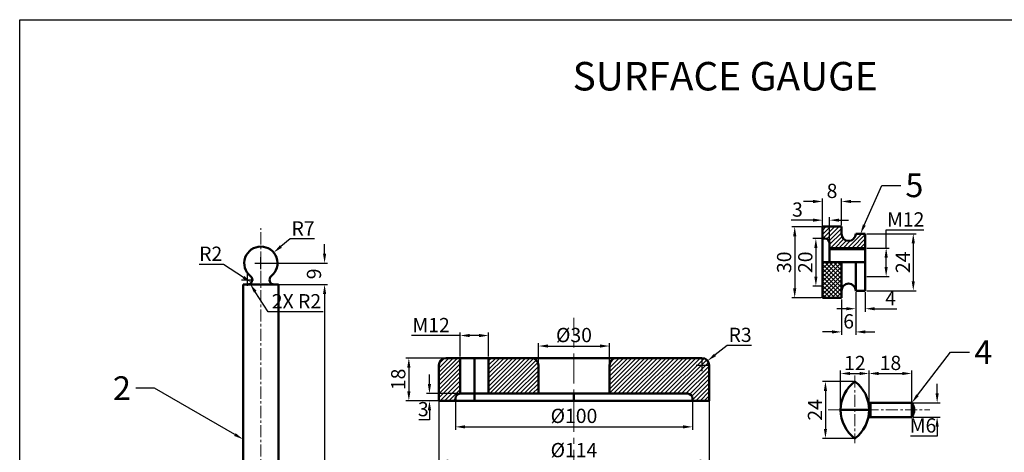
# Model space of a CAD drawing. Units: millimetres. Extents: x -65 to 576, y -103 to 374.
# Tile 3 of 4: x -65 to 351, y 192 to 374. Entities that reach past the tile are written whole.
import ezdxf
from ezdxf import colors
from ezdxf.entities.mleader import LeaderData, LeaderLine
from ezdxf.math import Vec2, Vec3

# ---------------------------------------------------------------- set-up
doc = ezdxf.new("R2010")
doc.units = ezdxf.units.MM
doc.header["$LTSCALE"] = 0.4
doc.linetypes.add('CENTER', pattern=[50.8, 31.75, -6.35, 6.35, -6.35])
for name, color, linetype, lineweight in [('M-CNTR', 4, 'CENTER', 18), ('M-DIMS', 2, 'Continuous', 25), ('M-HATC', 8, 'Continuous', 18), ('M-OUTL', 7, 'Continuous', 50), ('M-TEXT', 3, 'Continuous', 25), ('M-TTLB', 7, 'Continuous', 25)]:
    doc.layers.add(name, color=color, linetype=linetype, lineweight=lineweight)
doc.styles.get("Standard").update_dxf_attribs({"font": 'arial.ttf'})
doc.dimstyles.new('ISO-25', dxfattribs={"dimtxt": 6, "dimasz": 4, "dimexe": 1.25, "dimexo": 0.625, "dimtad": 1, "dimtoh": 1, "dimtxsty": 'Standard', "dimcen": 2.5, "dimadec": 0, "dimazin": 0, "dimtfac": 1, "dimtofl": 0, "dimtmove": 0, "dimatfit": 3, "dimfxl": 1, "dimarcsym": 0})

# ---------------------------------------------------------------- blocks, each defined once
blk = doc.blocks.new('*D1')
at = {"layer": 'Defpoints', "color": 0, "ltscale": 0.4, "transparency": 16777216}
for p in [(112.15, 220.83), (226.15, 220.83), (226.15, 187.9)]:
    blk.add_point(p, dxfattribs=at)
at = {"layer": 'M-DIMS', "color": 0, "lineweight": -2, "ltscale": 0.4, "transparency": 16777216}
for p, q in [((112.15, 220.2), (112.15, 186.65)), ((226.15, 220.2), (226.15, 186.65)), ((116.15, 187.9), (222.15, 187.9))]:
    blk.add_line(p, q, dxfattribs=at)
at = {"layer": 'M-DIMS', "color": 0, "ltscale": 0.4, "transparency": 16777216}
for points in [[(116.15, 188.57), (116.15, 187.24), (112.15, 187.9)], [(222.15, 188.57), (222.15, 187.24), (226.15, 187.9)]]:
    blk.add_solid(points, dxfattribs=at)
at = {"layer": 'M-DIMS', "color": 0, "ltscale": 0.4, "transparency": 16777216, "insert": (169.15, 191.76), "char_height": 6, "attachment_point": 5}
blk.add_mtext('%%C114', dxfattribs=at)
blk = doc.blocks.new('*D2')
at = {"layer": 'Defpoints', "color": 0, "ltscale": 0.4, "transparency": 16777216}
for p in [(119.15, 213.33), (219.15, 213.33), (219.15, 202.34)]:
    blk.add_point(p, dxfattribs=at)
at = {"layer": 'M-DIMS', "color": 0, "lineweight": -2, "ltscale": 0.4, "transparency": 16777216}
for p, q in [((119.15, 212.7), (119.15, 201.09)), ((219.15, 212.7), (219.15, 201.09)), ((123.15, 202.34), (215.15, 202.34))]:
    blk.add_line(p, q, dxfattribs=at)
at = {"layer": 'M-DIMS', "color": 0, "ltscale": 0.4, "transparency": 16777216}
for points in [[(123.15, 203), (123.15, 201.67), (119.15, 202.34)], [(215.15, 203), (215.15, 201.67), (219.15, 202.34)]]:
    blk.add_solid(points, dxfattribs=at)
at = {"layer": 'M-DIMS', "color": 0, "ltscale": 0.4, "transparency": 16777216, "insert": (169.15, 206.19), "char_height": 6, "attachment_point": 5}
blk.add_mtext('%%C100', dxfattribs=at)
blk = doc.blocks.new('*D3')
at = {"layer": 'Defpoints', "color": 0, "ltscale": 0.4, "transparency": 16777216}
for p in [(184.15, 236.39), (154.15, 222.33), (184.15, 222.33)]:
    blk.add_point(p, dxfattribs=at)
at = {"layer": 'M-DIMS', "color": 0, "lineweight": -2, "ltscale": 0.4, "transparency": 16777216}
for p, q in [((154.15, 222.95), (154.15, 237.64)), ((184.15, 222.95), (184.15, 237.64)), ((158.15, 236.39), (180.15, 236.39))]:
    blk.add_line(p, q, dxfattribs=at)
at = {"layer": 'M-DIMS', "color": 0, "ltscale": 0.4, "transparency": 16777216}
for points in [[(158.15, 237.05), (158.15, 235.72), (154.15, 236.39)], [(180.15, 237.05), (180.15, 235.72), (184.15, 236.39)]]:
    blk.add_solid(points, dxfattribs=at)
at = {"layer": 'M-DIMS', "color": 0, "ltscale": 0.4, "transparency": 16777216, "insert": (169.15, 240.24), "char_height": 6, "attachment_point": 5}
blk.add_mtext('%%C30', dxfattribs=at)
blk = doc.blocks.new('*D4')
at = {"layer": 'Defpoints', "color": 0, "ltscale": 0.4, "transparency": 16777216}
for p in [(133.15, 240.8), (121.15, 231.33), (133.15, 231.33)]:
    blk.add_point(p, dxfattribs=at)
at = {"layer": 'M-DIMS', "color": 0, "lineweight": -2, "ltscale": 0.4, "transparency": 16777216}
for p, q in [((121.15, 231.95), (121.15, 242.05)), ((133.15, 231.95), (133.15, 242.05)), ((121.15, 240.8), (100.65, 240.8)), ((129.15, 240.8), (125.15, 240.8))]:
    blk.add_line(p, q, dxfattribs=at)
at = {"layer": 'M-DIMS', "color": 0, "ltscale": 0.4, "transparency": 16777216}
for points in [[(125.15, 241.47), (125.15, 240.14), (121.15, 240.8)], [(129.15, 241.47), (129.15, 240.14), (133.15, 240.8)]]:
    blk.add_solid(points, dxfattribs=at)
at = {"layer": 'M-DIMS', "color": 0, "ltscale": 0.4, "transparency": 16777216, "insert": (108.9, 244.44), "char_height": 6, "attachment_point": 5}
blk.add_mtext('M12', dxfattribs=at)
blk = doc.blocks.new('*D5')
at = {"layer": 'Defpoints', "color": 0, "ltscale": 0.4, "transparency": 16777216}
for p in [(115.15, 231.33), (99.51, 213.33), (115.15, 213.33)]:
    blk.add_point(p, dxfattribs=at)
at = {"layer": 'M-DIMS', "color": 0, "lineweight": -2, "ltscale": 0.4, "transparency": 16777216}
for p, q in [((114.52, 231.33), (98.26, 231.33)), ((99.51, 227.33), (99.51, 217.33)), ((114.52, 213.33), (98.26, 213.33))]:
    blk.add_line(p, q, dxfattribs=at)
at = {"layer": 'M-DIMS', "color": 0, "ltscale": 0.4, "transparency": 16777216}
for points in [[(98.84, 227.33), (100.18, 227.33), (99.51, 231.33)], [(98.84, 217.33), (100.18, 217.33), (99.51, 213.33)]]:
    blk.add_solid(points, dxfattribs=at)
at = {"layer": 'M-DIMS', "color": 0, "ltscale": 0.4, "transparency": 16777216, "insert": (95.82, 222.33), "char_height": 6, "attachment_point": 5, "rotation": 90}
blk.add_mtext('18', dxfattribs=at)
blk = doc.blocks.new('*D6')
at = {"layer": 'Defpoints', "color": 0, "ltscale": 0.4, "transparency": 16777216}
for p in [(125.51, 216.33), (108.2, 213.33), (125.51, 213.33)]:
    blk.add_point(p, dxfattribs=at)
at = {"layer": 'M-DIMS', "color": 0, "lineweight": -2, "ltscale": 0.4, "transparency": 16777216}
for p, q in [((108.2, 220.33), (108.2, 224.33)), ((124.88, 216.33), (106.95, 216.33)), ((124.88, 213.33), (106.95, 213.33)), ((108.2, 209.33), (108.2, 205.33)), ((108.2, 205.33), (103.65, 205.33))]:
    blk.add_line(p, q, dxfattribs=at)
at = {"layer": 'M-DIMS', "color": 0, "ltscale": 0.4, "transparency": 16777216}
for points in [[(107.53, 220.33), (108.87, 220.33), (108.2, 216.33)], [(107.53, 209.33), (108.87, 209.33), (108.2, 213.33)]]:
    blk.add_solid(points, dxfattribs=at)
at = {"layer": 'M-DIMS', "color": 0, "ltscale": 0.4, "transparency": 16777216, "insert": (105.61, 209.02), "char_height": 6, "attachment_point": 5}
blk.add_mtext('3', dxfattribs=at)
blk = doc.blocks.new('*D7')
at = {"layer": 'Defpoints', "color": 0, "ltscale": 0.4, "transparency": 16777216}
for p in [(225.51, 230.18), (223.15, 228.33)]:
    blk.add_point(p, dxfattribs=at)
at = {"layer": 'M-DIMS', "color": 0, "lineweight": -2, "ltscale": 0.4, "transparency": 16777216}
for p, q in [((233.76, 236.63), (228.66, 232.64)), ((244.06, 236.63), (233.76, 236.63)), ((223.15, 225.83), (223.15, 230.83)), ((220.65, 228.33), (225.65, 228.33))]:
    blk.add_line(p, q, dxfattribs=at)
at = {"layer": 'M-DIMS', "color": 0, "ltscale": 0.4, "transparency": 16777216}
blk.add_solid([(228.25, 233.16), (229.07, 232.11), (225.51, 230.18)], dxfattribs=at)
at = {"layer": 'M-DIMS', "color": 0, "ltscale": 0.4, "transparency": 16777216, "insert": (239.22, 240.32), "char_height": 6, "attachment_point": 5}
blk.add_mtext('R3', dxfattribs=at)
blk = doc.blocks.new('*D12')
at = {"layer": 'Defpoints', "color": 0, "ltscale": 0.4, "transparency": 16777216}
for p in [(44.59, 262.28), (46.09, -30.72), (63.96, -30.72)]:
    blk.add_point(p, dxfattribs=at)
at = {"layer": 'M-DIMS', "color": 0, "lineweight": -2, "ltscale": 0.4, "transparency": 16777216}
for p, q in [((45.22, 262.28), (65.21, 262.28)), ((63.96, 258.28), (63.96, -26.72)), ((46.72, -30.72), (65.21, -30.72))]:
    blk.add_line(p, q, dxfattribs=at)
at = {"layer": 'M-DIMS', "color": 0, "ltscale": 0.4, "transparency": 16777216}
for points in [[(63.29, 258.28), (64.63, 258.28), (63.96, 262.28)], [(63.29, -26.72), (64.63, -26.72), (63.96, -30.72)]]:
    blk.add_solid(points, dxfattribs=at)
at = {"layer": 'M-DIMS', "color": 0, "ltscale": 0.4, "transparency": 16777216, "insert": (60.27, 115.78), "char_height": 6, "attachment_point": 5, "rotation": 90}
blk.add_mtext('293', dxfattribs=at)
blk = doc.blocks.new('*D17')
at = {"layer": 'Defpoints', "color": 0, "ltscale": 0.4, "transparency": 16777216}
for p in [(37.09, 271.28), (37.09, 262.28), (63.96, 262.28)]:
    blk.add_point(p, dxfattribs=at)
at = {"layer": 'M-DIMS', "color": 0, "lineweight": -2, "ltscale": 0.4, "transparency": 16777216}
for p, q in [((63.96, 275.28), (63.96, 279.28)), ((37.72, 271.28), (65.21, 271.28)), ((37.72, 262.28), (65.21, 262.28)), ((63.96, 258.28), (63.96, 254.28))]:
    blk.add_line(p, q, dxfattribs=at)
at = {"layer": 'M-DIMS', "color": 0, "ltscale": 0.4, "transparency": 16777216}
for points in [[(63.29, 275.28), (64.63, 275.28), (63.96, 271.28)], [(63.29, 258.28), (64.63, 258.28), (63.96, 262.28)]]:
    blk.add_solid(points, dxfattribs=at)
at = {"layer": 'M-DIMS', "color": 0, "ltscale": 0.4, "transparency": 16777216, "insert": (60.27, 266.78), "char_height": 6, "attachment_point": 5, "rotation": 90}
blk.add_mtext('9', dxfattribs=at)
blk = doc.blocks.new('*D18')
at = {"layer": 'Defpoints', "color": 0, "ltscale": 0.4, "transparency": 16777216}
for p in [(31.44, 264.28), (33.11, 263.19)]:
    blk.add_point(p, dxfattribs=at)
at = {"layer": 'M-DIMS', "color": 0, "lineweight": -2, "ltscale": 0.4, "transparency": 16777216}
for p, q in [((11.13, 270.85), (21.37, 270.85)), ((21.37, 270.85), (29.76, 265.37))]:
    blk.add_line(p, q, dxfattribs=at)
at = {"layer": 'M-DIMS', "color": 0, "ltscale": 0.4, "transparency": 16777216}
blk.add_solid([(30.13, 265.93), (29.4, 264.82), (33.11, 263.19)], dxfattribs=at)
at = {"layer": 'M-DIMS', "color": 0, "ltscale": 0.4, "transparency": 16777216, "insert": (15.94, 274.49), "char_height": 6, "attachment_point": 5}
blk.add_mtext('R2', dxfattribs=at)
blk = doc.blocks.new('*D19')
at = {"layer": 'Defpoints', "color": 0, "ltscale": 0.4, "transparency": 16777216}
for p in [(42.48, 275.75), (37.09, 271.28)]:
    blk.add_point(p, dxfattribs=at)
at = {"layer": 'M-DIMS', "color": 0, "lineweight": -2, "ltscale": 0.4, "transparency": 16777216}
for p, q in [((49.42, 281.51), (45.56, 278.3)), ((59.72, 281.51), (49.42, 281.51)), ((34.59, 271.28), (39.59, 271.28)), ((37.09, 268.78), (37.09, 273.78))]:
    blk.add_line(p, q, dxfattribs=at)
at = {"layer": 'M-DIMS', "color": 0, "ltscale": 0.4, "transparency": 16777216}
blk.add_solid([(45.13, 278.82), (45.98, 277.79), (42.48, 275.75)], dxfattribs=at)
at = {"layer": 'M-DIMS', "color": 0, "ltscale": 0.4, "transparency": 16777216, "insert": (54.89, 285.14), "char_height": 6, "attachment_point": 5}
blk.add_mtext('R7', dxfattribs=at)
blk = doc.blocks.new('*D20')
at = {"layer": 'Defpoints', "color": 0, "ltscale": 0.4, "transparency": 16777216}
for p in [(293.63, 224.81), (281.63, 209.48), (293.63, 209.48)]:
    blk.add_point(p, dxfattribs=at)
at = {"layer": 'M-DIMS', "color": 0, "lineweight": -2, "ltscale": 0.4, "transparency": 16777216}
for p, q in [((281.63, 210.1), (281.63, 226.06)), ((285.63, 224.81), (289.63, 224.81)), ((293.63, 210.1), (293.63, 226.06))]:
    blk.add_line(p, q, dxfattribs=at)
at = {"layer": 'M-DIMS', "color": 0, "ltscale": 0.4, "transparency": 16777216}
for points in [[(285.63, 225.48), (285.63, 224.15), (281.63, 224.81)], [(289.63, 225.48), (289.63, 224.15), (293.63, 224.81)]]:
    blk.add_solid(points, dxfattribs=at)
at = {"layer": 'M-DIMS', "color": 0, "ltscale": 0.4, "transparency": 16777216, "insert": (287.63, 228.45), "char_height": 6, "attachment_point": 5}
blk.add_mtext('12', dxfattribs=at)
blk = doc.blocks.new('*D21')
at = {"layer": 'Defpoints', "color": 0, "ltscale": 0.4, "transparency": 16777216}
for p in [(287.63, 221.48), (275.22, 197.48), (287.63, 197.48)]:
    blk.add_point(p, dxfattribs=at)
at = {"layer": 'M-DIMS', "color": 0, "lineweight": -2, "ltscale": 0.4, "transparency": 16777216}
for p, q in [((287, 221.48), (273.97, 221.48)), ((275.22, 217.48), (275.22, 201.48)), ((287, 197.48), (273.97, 197.48))]:
    blk.add_line(p, q, dxfattribs=at)
at = {"layer": 'M-DIMS', "color": 0, "ltscale": 0.4, "transparency": 16777216}
for points in [[(274.55, 217.48), (275.88, 217.48), (275.22, 221.48)], [(274.55, 201.48), (275.88, 201.48), (275.22, 197.48)]]:
    blk.add_solid(points, dxfattribs=at)
at = {"layer": 'M-DIMS', "color": 0, "ltscale": 0.4, "transparency": 16777216, "insert": (271.58, 209.48), "char_height": 6, "attachment_point": 5, "rotation": 90}
blk.add_mtext('24', dxfattribs=at)
blk = doc.blocks.new('*D22')
at = {"layer": 'Defpoints', "color": 0, "ltscale": 0.4, "transparency": 16777216}
for p in [(311.63, 212.48), (311.63, 206.48), (322.32, 206.48)]:
    blk.add_point(p, dxfattribs=at)
at = {"layer": 'M-DIMS', "color": 0, "lineweight": -2, "ltscale": 0.4, "transparency": 16777216}
for p, q in [((322.32, 216.48), (322.32, 220.48)), ((312.25, 212.48), (323.57, 212.48)), ((312.25, 206.48), (323.57, 206.48)), ((322.32, 202.48), (322.32, 198.48)), ((322.32, 198.48), (311.06, 198.48))]:
    blk.add_line(p, q, dxfattribs=at)
at = {"layer": 'M-DIMS', "color": 0, "ltscale": 0.4, "transparency": 16777216}
for points in [[(321.65, 216.48), (322.99, 216.48), (322.32, 212.48)], [(321.65, 202.48), (322.99, 202.48), (322.32, 206.48)]]:
    blk.add_solid(points, dxfattribs=at)
at = {"layer": 'M-DIMS', "color": 0, "ltscale": 0.4, "transparency": 16777216, "insert": (316.38, 202.16), "char_height": 6, "attachment_point": 5}
blk.add_mtext('M6', dxfattribs=at)
blk = doc.blocks.new('*D23')
at = {"layer": 'Defpoints', "color": 0, "ltscale": 0.4, "transparency": 16777216}
for p in [(311.63, 224.81), (293.63, 209.83), (311.63, 209.48)]:
    blk.add_point(p, dxfattribs=at)
at = {"layer": 'M-DIMS', "color": 0, "lineweight": -2, "ltscale": 0.4, "transparency": 16777216}
for p, q in [((293.63, 210.45), (293.63, 226.06)), ((297.63, 224.81), (307.63, 224.81)), ((311.63, 210.1), (311.63, 226.06))]:
    blk.add_line(p, q, dxfattribs=at)
at = {"layer": 'M-DIMS', "color": 0, "ltscale": 0.4, "transparency": 16777216}
for points in [[(297.63, 225.48), (297.63, 224.15), (293.63, 224.81)], [(307.63, 225.48), (307.63, 224.15), (311.63, 224.81)]]:
    blk.add_solid(points, dxfattribs=at)
at = {"layer": 'M-DIMS', "color": 0, "ltscale": 0.4, "transparency": 16777216, "insert": (302.63, 228.5), "char_height": 6, "attachment_point": 5}
blk.add_mtext('18', dxfattribs=at)
blk = doc.blocks.new('*D46')
at = {"layer": 'Defpoints', "color": 0, "ltscale": 0.4, "transparency": 16777216}
for p in [(273.99, 286.66), (262.25, 256.66), (273.99, 256.66)]:
    blk.add_point(p, dxfattribs=at)
at = {"layer": 'M-DIMS', "color": 0, "lineweight": -2, "ltscale": 0.4, "transparency": 16777216}
for p, q in [((273.36, 286.66), (261, 286.66)), ((262.25, 282.66), (262.25, 260.66)), ((273.36, 256.66), (261, 256.66))]:
    blk.add_line(p, q, dxfattribs=at)
at = {"layer": 'M-DIMS', "color": 0, "ltscale": 0.4, "transparency": 16777216}
for points in [[(261.59, 282.66), (262.92, 282.66), (262.25, 286.66)], [(261.59, 260.66), (262.92, 260.66), (262.25, 256.66)]]:
    blk.add_solid(points, dxfattribs=at)
at = {"layer": 'M-DIMS', "color": 0, "ltscale": 0.4, "transparency": 16777216, "insert": (258.56, 271.66), "char_height": 6, "attachment_point": 5, "rotation": 90}
blk.add_mtext('30', dxfattribs=at)
blk = doc.blocks.new('*D47')
at = {"layer": 'Defpoints', "color": 0, "ltscale": 0.4, "transparency": 16777216}
for p in [(273.99, 281.66), (271.18, 261.66), (274.49, 261.66)]:
    blk.add_point(p, dxfattribs=at)
at = {"layer": 'M-DIMS', "color": 0, "lineweight": -2, "ltscale": 0.4, "transparency": 16777216}
for p, q in [((273.36, 281.66), (269.93, 281.66)), ((271.18, 277.66), (271.18, 265.66)), ((273.86, 261.66), (269.93, 261.66))]:
    blk.add_line(p, q, dxfattribs=at)
at = {"layer": 'M-DIMS', "color": 0, "ltscale": 0.4, "transparency": 16777216}
for points in [[(270.51, 277.66), (271.85, 277.66), (271.18, 281.66)], [(270.51, 265.66), (271.85, 265.66), (271.18, 261.66)]]:
    blk.add_solid(points, dxfattribs=at)
at = {"layer": 'M-DIMS', "color": 0, "ltscale": 0.4, "transparency": 16777216, "insert": (267.49, 271.66), "char_height": 6, "attachment_point": 5, "rotation": 90}
blk.add_mtext('20', dxfattribs=at)
blk = doc.blocks.new('*D48')
at = {"layer": 'Defpoints', "color": 0, "ltscale": 0.4, "transparency": 16777216}
for p in [(281.99, 297.27), (273.99, 286.66), (281.99, 286.66)]:
    blk.add_point(p, dxfattribs=at)
at = {"layer": 'M-DIMS', "color": 0, "lineweight": -2, "ltscale": 0.4, "transparency": 16777216}
for p, q in [((269.99, 297.27), (265.99, 297.27)), ((273.99, 287.29), (273.99, 298.52)), ((281.99, 287.29), (281.99, 298.52)), ((285.99, 297.27), (289.99, 297.27))]:
    blk.add_line(p, q, dxfattribs=at)
at = {"layer": 'M-DIMS', "color": 0, "ltscale": 0.4, "transparency": 16777216}
for points in [[(269.99, 297.93), (269.99, 296.6), (273.99, 297.27)], [(285.99, 297.93), (285.99, 296.6), (281.99, 297.27)]]:
    blk.add_solid(points, dxfattribs=at)
at = {"layer": 'M-DIMS', "color": 0, "ltscale": 0.4, "transparency": 16777216, "insert": (277.99, 300.95), "char_height": 6, "attachment_point": 5}
blk.add_mtext('8', dxfattribs=at)
blk = doc.blocks.new('*D49')
at = {"layer": 'Defpoints', "color": 0, "ltscale": 0.4, "transparency": 16777216}
for p in [(276.99, 289.4), (273.99, 277.61), (276.99, 277.61)]:
    blk.add_point(p, dxfattribs=at)
at = {"layer": 'M-DIMS', "color": 0, "lineweight": -2, "ltscale": 0.4, "transparency": 16777216}
for p, q in [((269.99, 289.4), (260.81, 289.4)), ((273.99, 278.24), (273.99, 290.65)), ((276.99, 278.24), (276.99, 290.65)), ((280.99, 289.4), (284.99, 289.4))]:
    blk.add_line(p, q, dxfattribs=at)
at = {"layer": 'M-DIMS', "color": 0, "ltscale": 0.4, "transparency": 16777216}
for points in [[(269.99, 290.07), (269.99, 288.74), (273.99, 289.4)], [(280.99, 290.07), (280.99, 288.74), (276.99, 289.4)]]:
    blk.add_solid(points, dxfattribs=at)
at = {"layer": 'M-DIMS', "color": 0, "ltscale": 0.4, "transparency": 16777216, "insert": (263.4, 293.09), "char_height": 6, "attachment_point": 5}
blk.add_mtext('3', dxfattribs=at)
blk = doc.blocks.new('*D50')
at = {"layer": 'Defpoints', "color": 0, "ltscale": 0.4, "transparency": 16777216}
for p in [(291.99, 277.66), (300.82, 277.66), (291.99, 265.66)]:
    blk.add_point(p, dxfattribs=at)
at = {"layer": 'M-DIMS', "color": 0, "lineweight": -2, "ltscale": 0.4, "transparency": 16777216}
for p, q in [((300.82, 277.66), (300.82, 285.3)), ((300.82, 285.3), (316.69, 285.3)), ((292.61, 277.66), (302.07, 277.66)), ((300.82, 269.66), (300.82, 273.66)), ((292.61, 265.66), (302.07, 265.66))]:
    blk.add_line(p, q, dxfattribs=at)
at = {"layer": 'M-DIMS', "color": 0, "ltscale": 0.4, "transparency": 16777216}
for points in [[(300.15, 273.66), (301.49, 273.66), (300.82, 277.66)], [(300.15, 269.66), (301.49, 269.66), (300.82, 265.66)]]:
    blk.add_solid(points, dxfattribs=at)
at = {"layer": 'M-DIMS', "color": 0, "ltscale": 0.4, "transparency": 16777216, "insert": (309.06, 288.94), "char_height": 6, "attachment_point": 5}
blk.add_mtext('M12', dxfattribs=at)
blk = doc.blocks.new('*D51')
at = {"layer": 'Defpoints', "color": 0, "ltscale": 0.4, "transparency": 16777216}
for p in [(291.99, 283.66), (291.99, 259.66), (312.26, 259.66)]:
    blk.add_point(p, dxfattribs=at)
at = {"layer": 'M-DIMS', "color": 0, "lineweight": -2, "ltscale": 0.4, "transparency": 16777216}
for p, q in [((292.61, 283.66), (313.51, 283.66)), ((312.26, 279.66), (312.26, 263.66)), ((292.61, 259.66), (313.51, 259.66))]:
    blk.add_line(p, q, dxfattribs=at)
at = {"layer": 'M-DIMS', "color": 0, "ltscale": 0.4, "transparency": 16777216}
for points in [[(311.59, 279.66), (312.93, 279.66), (312.26, 283.66)], [(311.59, 263.66), (312.93, 263.66), (312.26, 259.66)]]:
    blk.add_solid(points, dxfattribs=at)
at = {"layer": 'M-DIMS', "color": 0, "ltscale": 0.4, "transparency": 16777216, "insert": (308.62, 271.66), "char_height": 6, "attachment_point": 5, "rotation": 90}
blk.add_mtext('24', dxfattribs=at)
blk = doc.blocks.new('*D52')
at = {"layer": 'Defpoints', "color": 0, "ltscale": 0.4, "transparency": 16777216}
for p in [(287.99, 259.66), (281.99, 256.66), (287.99, 242.33)]:
    blk.add_point(p, dxfattribs=at)
at = {"layer": 'M-DIMS', "color": 0, "lineweight": -2, "ltscale": 0.4, "transparency": 16777216}
for p, q in [((287.99, 259.04), (287.99, 241.08)), ((281.99, 256.04), (281.99, 241.08)), ((277.99, 242.33), (273.99, 242.33)), ((291.99, 242.33), (295.99, 242.33))]:
    blk.add_line(p, q, dxfattribs=at)
at = {"layer": 'M-DIMS', "color": 0, "ltscale": 0.4, "transparency": 16777216}
for points in [[(277.99, 243), (277.99, 241.66), (281.99, 242.33)], [(291.99, 243), (291.99, 241.66), (287.99, 242.33)]]:
    blk.add_solid(points, dxfattribs=at)
at = {"layer": 'M-DIMS', "color": 0, "ltscale": 0.4, "transparency": 16777216, "insert": (284.99, 246.02), "char_height": 6, "attachment_point": 5}
blk.add_mtext('6', dxfattribs=at)
blk = doc.blocks.new('*D53')
at = {"layer": 'Defpoints', "color": 0, "ltscale": 0.4, "transparency": 16777216}
for p in [(287.99, 259.66), (291.99, 259.66), (291.99, 252.1)]:
    blk.add_point(p, dxfattribs=at)
at = {"layer": 'M-DIMS', "color": 0, "lineweight": -2, "ltscale": 0.4, "transparency": 16777216}
for p, q in [((287.99, 259.04), (287.99, 250.85)), ((291.99, 259.04), (291.99, 250.85)), ((283.99, 252.1), (279.99, 252.1)), ((295.99, 252.1), (305.39, 252.1))]:
    blk.add_line(p, q, dxfattribs=at)
at = {"layer": 'M-DIMS', "color": 0, "ltscale": 0.4, "transparency": 16777216}
for points in [[(283.99, 252.76), (283.99, 251.43), (287.99, 252.1)], [(295.99, 252.76), (295.99, 251.43), (291.99, 252.1)]]:
    blk.add_solid(points, dxfattribs=at)
at = {"layer": 'M-DIMS', "color": 0, "ltscale": 0.4, "transparency": 16777216, "insert": (302.69, 255.72), "char_height": 6, "attachment_point": 5}
blk.add_mtext('4', dxfattribs=at)
blk = doc.blocks.new('*D55')
at = {"layer": 'Defpoints', "color": 0, "ltscale": 0.4, "transparency": 16777216}
for p in [(31.44, 264.28), (32.53, 262.6)]:
    blk.add_point(p, dxfattribs=at)
at = {"layer": 'M-DIMS', "color": 0, "lineweight": -2, "ltscale": 0.4, "transparency": 16777216}
for p, q in [((31.44, 261.78), (31.44, 266.78)), ((28.94, 264.28), (33.94, 264.28)), ((40.18, 250.84), (34.71, 259.25)), ((63.41, 250.84), (40.18, 250.84))]:
    blk.add_line(p, q, dxfattribs=at)
at = {"layer": 'M-DIMS', "color": 0, "ltscale": 0.4, "transparency": 16777216}
blk.add_solid([(35.27, 259.61), (34.15, 258.89), (32.53, 262.6)], dxfattribs=at)
at = {"layer": 'M-DIMS', "color": 0, "ltscale": 0.4, "transparency": 16777216, "insert": (52.11, 254.48), "char_height": 6, "attachment_point": 5}
blk.add_mtext('2X R2', dxfattribs=at)

msp = doc.modelspace()

# ---------------------------------------------------------------- hatches: boundary and pattern name
at = {"layer": 'M-HATC', "ltscale": 0.4}
h = msp.add_hatch(dxfattribs=at)
h.set_pattern_fill('ANSI31', color=256, scale=0.4)
h.set_pattern_definition([(45, (-264.7633, 186.3798), (-0.8980256, 0.8980256), [])])
h.paths.add_polyline_path([(281.989, 283.665), (281.989, 286.665), (273.989, 286.665), (273.989, 281.665), (274.989, 281.665, -0.4142136), (276.989, 279.665), (276.989, 277.665), (291.989, 277.665), (291.989, 283.665), (287.989, 283.665, -1)])
h = msp.add_hatch(dxfattribs=at)
h.set_pattern_fill('ANSI37', color=256, scale=0.4)
h.set_pattern_definition([(45, (-264.7633, 186.3798), (-0.8980256, 0.8980256), []), (135, (-264.7633, 186.3798), (-0.8980256, -0.8980256), [])])
h.paths.add_polyline_path([(273.989, 256.665), (281.989, 256.665), (281.989, 271.665), (273.989, 271.665)])
h = msp.add_hatch(dxfattribs=at)
h.set_pattern_fill('ANSI31', color=256, scale=0.4)
h.paths.add_polyline_path([(226.146, 228.328, 0.4142136), (223.146, 231.328), (187.146, 231.328, 0.4142136), (184.146, 228.328), (184.146, 216.328), (217.146, 216.328, -0.4142136), (219.146, 214.328), (219.146, 213.328), (226.146, 213.328)])
h.paths.add_polyline_path([(154.146, 228.328, 0.4142136), (151.146, 231.328), (133.146, 231.328), (133.146, 216.328), (154.146, 216.328)])
h.paths.add_polyline_path([(121.146, 231.328), (115.146, 231.328, 0.4142136), (112.146, 228.328), (112.146, 213.328), (119.146, 213.328), (119.146, 214.328, -0.4142136), (121.146, 216.328)])

# ---------------------------------------------------------------- linework, layer by layer
at = {"layer": 'M-CNTR', "ltscale": 0.4}
for p, q in [((37.094, -62.16), (37.094, 286.009)), ((287.627, 223.945), (287.627, 195.492)), ((276.321, 209.476), (319.197, 209.476))]:
    msp.add_line(p, q, dxfattribs=at)
at = {"layer": 'M-CNTR'}
msp.add_line((169.146, 118.958), (169.146, 248.195), dxfattribs=at)
at = {"layer": 'M-OUTL', "ltscale": 0.4}
for p, q in [((273.989, 286.665), (273.989, 271.665)), ((281.989, 286.665), (273.989, 286.665)), ((281.989, 283.665), (281.989, 286.665)), ((291.989, 283.665), (287.989, 283.665)), ((291.989, 283.665), (291.989, 271.665)), ((274.989, 281.665), (273.989, 281.665)), ((276.989, 279.665), (276.989, 271.665)), ((276.989, 277.665), (291.989, 277.665)), ((276.989, 277.165), (291.989, 277.165)), ((273.989, 271.665), (291.989, 271.665)), ((276.989, 271.665), (273.989, 271.665)), ((273.989, 256.665), (273.989, 271.665)), ((276.989, 271.665), (273.989, 271.665)), ((281.989, 256.665), (281.989, 271.665)), ((287.989, 259.665), (287.989, 271.665)), ((291.989, 259.665), (291.989, 271.665)), ((29.594, 262.281), (29.594, 131.923)), ((29.594, 262.281), (31.437, 262.281)), ((31.437, 262.281), (44.594, 262.281)), ((44.594, 262.281), (44.594, 131.923)), ((281.989, 259.665), (281.989, 256.665)), ((291.989, 259.665), (287.989, 259.665)), ((281.989, 256.665), (273.989, 256.665)), ((311.627, 212.476), (293.324, 212.476)), ((294.173, 212.476), (294.173, 206.476)), ((311.627, 209.476), (311.627, 212.476)), ((281.627, 209.476), (293.627, 209.476)), ((311.627, 209.476), (311.627, 206.476)), ((311.627, 206.476), (293.324, 206.476))]:
    msp.add_line(p, q, dxfattribs=at)
at = {"layer": 'M-OUTL'}
for p, q in [((115.146, 231.328), (187.146, 231.328)), ((121.146, 216.328), (121.146, 231.328)), ((127.146, 213.328), (127.146, 231.328)), ((133.146, 216.328), (133.146, 231.328)), ((187.146, 231.328), (223.146, 231.328)), ((112.146, 213.328), (112.146, 228.328)), ((154.146, 216.328), (154.146, 228.328)), ((184.146, 216.328), (184.146, 228.328)), ((226.146, 228.328), (226.146, 213.328)), ((217.146, 216.328), (121.146, 216.328)), ((169.146, 216.328), (169.146, 213.328)), ((226.146, 213.328), (112.146, 213.328)), ((119.146, 213.328), (119.146, 214.328)), ((119.146, 213.328), (119.146, 213.328)), ((219.146, 213.328), (219.146, 214.328)), ((219.146, 213.328), (219.146, 213.328))]:
    msp.add_line(p, q, dxfattribs=at)
at = {"layer": 'M-OUTL', "ltscale": 0.4}
for centre, radius, start, end in [((284.989, 283.665), 3, 180, 0), ((37.094, 271.281), 7, 308.94244, 231.05756), ((274.989, 279.665), 2, 0, 90), ((31.437, 264.281), 2, 270, 51.05756), ((42.751, 264.281), 2, 128.94244, 270), ((284.989, 259.665), 3, 0, 180), ((296.627, 209.476), 15, 126.8699, 233.1301), ((278.627, 209.476), 15, 306.8699, 53.1301), ((307.634, 209.476), 4.994, 323.07769, 36.92231)]:
    msp.add_arc(centre, radius, start, end, dxfattribs=at)
at = {"layer": 'M-OUTL'}
for centre, radius, start, end in [((115.146, 228.328), 3, 90, 180), ((151.146, 228.328), 3, 0, 90), ((187.146, 228.328), 3, 90, 180), ((223.146, 228.328), 3, 0, 90), ((121.146, 214.328), 2, 90, 180), ((217.146, 214.328), 2, 0, 90)]:
    msp.add_arc(centre, radius, start, end, dxfattribs=at)
at = {"layer": 'M-TTLB', "ltscale": 0.4}
msp.add_lwpolyline([(-64.629, 373.834), (576.345, 373.834), (576.345, -103.363), (-64.629, -103.363)], close=True, dxfattribs=at)

# ---------------------------------------------------------------- texts
at = {"layer": 'M-TEXT', "ltscale": 0.4, "insert": (156.13, 356.034), "char_height": 12, "attachment_point": 1}
msp.add_mtext_dynamic_manual_height_columns('\\pxqc;SURFACE GAUGE', width=153.60759, gutter_width=12.5, heights=[0], dxfattribs=at)

# ---------------------------------------------------------------- dimensions: what is measured, and where the dimension line sits
at = {"layer": 'M-DIMS', "ltscale": 0.4}
for base, p1, p2, picture, middle in [((281.989, 297.266), (273.989, 286.665), (281.989, 286.665), '*D48', (277.989, 300.954)), ((291.989, 252.097), (287.989, 259.665), (291.989, 259.665), '*D53', (302.689, 255.722)), ((293.627, 224.815), (281.627, 209.476), (293.627, 209.476), '*D20', (287.627, 228.452)), ((311.627, 224.815), (293.627, 209.827), (311.627, 209.476), '*D23', (302.627, 228.503))]:
    dim = msp.add_linear_dim(base=base, p1=p1, p2=p2, dimstyle='ISO-25', override={"dimclrd": 0, "dimclre": 0, "dimclrt": 0}, dxfattribs=at)
    dim.commit()
    dim.dimension.update_dxf_attribs({"geometry": picture, "text_midpoint": middle})
for base, p1, p2, picture, middle in [((276.989, 289.404), (273.989, 277.612), (276.989, 277.612), '*D49', (263.399, 289.404)), ((287.989, 242.33), (281.989, 256.665), (287.989, 259.665), '*D52', (284.989, 242.33))]:
    dim = msp.add_linear_dim(base=base, p1=p1, p2=p2, dimstyle='ISO-25', override={"dimclrd": 0, "dimclre": 0, "dimclrt": 0}, dxfattribs=at)
    dim.commit()
    dim.dimension.update_dxf_attribs({"geometry": picture, "text_midpoint": middle, "dimtype": 160})
dim = msp.add_linear_dim(base=(300.819, 277.665), p1=(291.989, 265.665), p2=(291.989, 277.665), angle=90, text='M<>', dimstyle='ISO-25', override={"dimclrd": 0, "dimclre": 0, "dimclrt": 0}, dxfattribs=at)
dim.commit()
dim.dimension.update_dxf_attribs({"geometry": '*D50', "text_midpoint": (309.064, 285.302), "dimtype": 160})
for center, mpoint, picture, middle in [((37.094, 271.281), (42.481, 275.751), '*D19', (54.887, 281.512)), ((31.437, 264.281), (33.112, 263.188), '*D18', (15.935, 270.853)), ((223.146, 228.328), (225.509, 230.176), '*D7', (239.222, 236.626))]:
    dim = msp.add_radius_dim(center=center, mpoint=mpoint, dimstyle='ISO-25', override={"dimclrd": 0, "dimclre": 0, "dimclrt": 0}, dxfattribs=at)
    dim.commit()
    dim.dimension.update_dxf_attribs({"geometry": picture, "text_midpoint": middle, "dimtype": 164})
for base, p1, p2, picture, middle in [((262.252, 256.665), (273.989, 286.665), (273.989, 256.665), '*D46', (258.561, 271.665)), ((312.26, 259.665), (291.989, 283.665), (291.989, 259.665), '*D51', (308.622, 271.665)), ((63.961, 262.281), (37.094, 271.281), (37.094, 262.281), '*D17', (60.273, 266.781)), ((271.18, 261.665), (273.989, 281.665), (274.489, 261.665), '*D47', (267.492, 271.665)), ((63.961, -30.719), (44.594, 262.281), (46.094, -30.719), '*D12', (60.271, 115.781)), ((99.51, 213.328), (115.146, 231.328), (115.146, 213.328), '*D5', (95.821, 222.328)), ((108.202, 213.328), (125.509, 216.328), (125.509, 213.328), '*D6', (105.612, 209.019)), ((275.218, 197.476), (287.627, 221.476), (287.627, 197.476), '*D21', (271.581, 209.476))]:
    dim = msp.add_linear_dim(base=base, p1=p1, p2=p2, angle=90, dimstyle='ISO-25', override={"dimclrd": 0, "dimclre": 0, "dimclrt": 0}, dxfattribs=at)
    dim.commit()
    dim.dimension.update_dxf_attribs({"geometry": picture, "text_midpoint": middle})
dim = msp.add_radius_dim(center=(31.437, 264.281), mpoint=(32.527, 262.604), text='2X <>', dimstyle='ISO-25', override={"dimdec": 0, "dimlfac": 1, "dimrnd": 0, "dimzin": 0, "dimdsep": 46, "dimlunit": 2}, dxfattribs=at)
dim.commit()
dim.dimension.update_dxf_attribs({"geometry": '*D55', "text_midpoint": (52.106, 254.484)})
for base, p1, p2, text, picture, middle in [((133.146, 240.803), (121.146, 231.328), (133.146, 231.328), 'M<>', '*D4', (108.9, 240.803)), ((226.146, 187.903), (112.146, 220.828), (226.146, 220.828), '%%C<>', '*D1', (169.146, 187.903)), ((219.146, 202.337), (119.146, 213.328), (219.146, 213.328), '%%C<>', '*D2', (169.146, 202.337))]:
    dim = msp.add_linear_dim(base=base, p1=p1, p2=p2, text=text, dimstyle='ISO-25', override={"dimclrd": 0, "dimclre": 0, "dimclrt": 0}, dxfattribs=at)
    dim.commit()
    dim.dimension.update_dxf_attribs({"geometry": picture, "text_midpoint": middle, "dimtype": 160})
dim = msp.add_linear_dim(base=(184.146, 236.388), p1=(154.146, 222.328), p2=(184.146, 222.328), text='%%C<>', dimstyle='ISO-25', override={"dimclrd": 0, "dimclre": 0, "dimclrt": 0}, dxfattribs=at)
dim.commit()
dim.dimension.update_dxf_attribs({"geometry": '*D3', "text_midpoint": (169.146, 240.244)})
dim = msp.add_linear_dim(base=(322.321, 206.476), p1=(311.627, 212.476), p2=(311.627, 206.476), angle=90, text='M<>', dimstyle='ISO-25', override={"dimclrd": 0, "dimclre": 0, "dimclrt": 0}, dxfattribs=at)
dim.commit()
dim.dimension.update_dxf_attribs({"geometry": '*D22', "text_midpoint": (316.377, 202.165)})

# ---------------------------------------------------------------- leaders
at = {"layer": 'M-TEXT', "ltscale": 0.4}
ml = msp.add_multileader_mtext('Standard', dxfattribs=at)
ml.set_content('5', color=256)
ml.set_leader_properties()
ml.build(insert=Vec2(0, 0))
ctx = ml.context
ctx.base_point, ctx.char_height, ctx.plane_origin = Vec3(306.942, 304.012), 10, Vec3(289.989, 283.665)
notes = []
notes.append((ctx, [(0, (1, 1, 0), (298.942, 304.012), (1, 0), 8, [(0, [(289.989, 283.665)], 0, [])])]))
ctx.mtext.insert, ctx.mtext.flow_direction = Vec3(308.942, 309.098), 5
ml = msp.add_multileader_mtext('Standard', dxfattribs=at)
ml.set_content('4', color=256)
ml.set_leader_properties()
ml.build(insert=Vec2(0, 0))
ctx = ml.context
ctx.base_point, ctx.char_height, ctx.plane_origin = Vec3(335.985, 233.798), 10, Vec3(311.627, 212.476)
notes.append((ctx, [(0, (1, 1, 0), (327.985, 233.798), (1, 0), 8, [(0, [(311.627, 212.476)], 0, [])])]))
ctx.mtext.insert, ctx.mtext.flow_direction = Vec3(337.985, 238.798), 5
ml = msp.add_multileader_mtext('Standard', dxfattribs=at)
ml.set_content('2', color=256)
ml.set_leader_properties()
ml.build(insert=Vec2(0, 0))
ctx = ml.context
ctx.base_point, ctx.char_height, ctx.plane_origin = Vec3(-26.334, 218.639), 10, Vec3(29.594, 197.102)
ctx.text_align_type = 2
notes.append((ctx, [(0, (1, 1, 0), (-7.71, 218.639), (-1, 0), 8, [(0, [(29.594, 197.102)], 0, [])])]))
ctx.mtext.insert, ctx.mtext.alignment, ctx.mtext.flow_direction = Vec3(-17.71, 223.639), 3, 5
for ctx, leaders in notes:
    for number, flags, end, landing, length, lines in leaders:
        leader = LeaderData()
        leader.index, (leader.has_last_leader_line, leader.has_dogleg_vector, leader.attachment_direction) = number, flags
        leader.last_leader_point, leader.dogleg_vector, leader.dogleg_length = Vec3(end), Vec3(landing), length
        for number, points, colour, breaks in lines:
            line = LeaderLine()
            line.index, line.vertices, line.color, line.breaks = number, Vec3.list(points), colors.encode_raw_color(colour), breaks
            leader.lines.append(line)
        ctx.leaders.append(leader)

doc.saveas('drawing.dxf')
